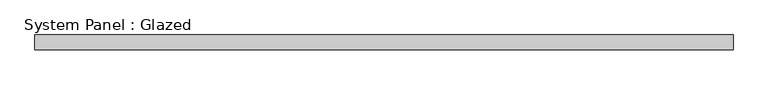
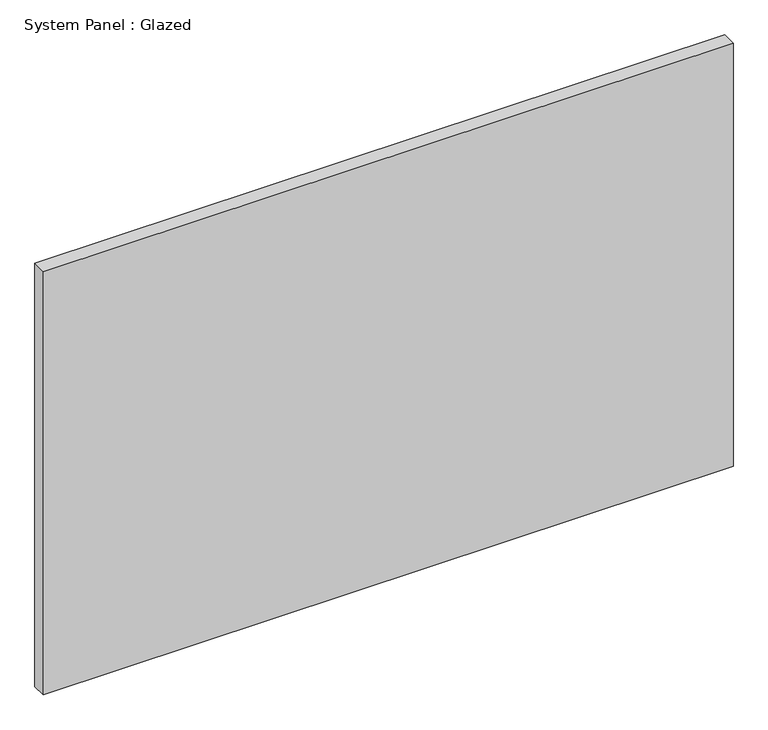
"""IFC4 building model written with IfcOpenShell, lengths in millimetres: plate geometry, System Panel : Glazed."""

from ifc_helpers import new_model, si_unit, origin, origin_with_axes, place, context, project, spatial, polyline, outline, extrude, source, transform, mapped, element, save


def system_panel_glazed_7a6fc0cf(model_context):
    return source(origin(), model_context, "Body", "SweptSolid", [
        extrude(outline(polyline([(604.6949353, 19.05), (-604.6949353, 19.05), (-604.6949353, 44.45), (604.6949353, 44.45), (604.6949353, 19.05)])), origin_with_axes(), (0.0, 0.0, 1.0), 784.5104839),
    ])


if __name__ == "__main__":
    model = new_model("IFC4")
    model_context = context("Model", 3, world=origin())
    ifc_project = project(units=[si_unit("LENGTHUNIT", "METRE", prefix="MILLI")], contexts=[model_context])
    site = spatial("IfcSite", under=ifc_project)
    building = spatial("IfcBuilding", under=site)
    placement = place(None, origin())
    system_panel_glazed_shape = system_panel_glazed_7a6fc0cf(model_context)
    element("IfcPlate", 1, ObjectType="System Panel : Glazed", at=placement, inside=building, context=model_context, shape_type="MappedRepresentation", body=[
        mapped(system_panel_glazed_shape, transform((0.0, 0.0, 0.0), x_axis=(1.0, 0.0, 0.0), y_axis=(0.0, 1.0, 0.0), z_axis=(0.0, 0.0, 1.0))),
    ])
    save(model, "model.ifc")

# Revit data of these elements
# Type "System Panel : Glazed"
#   Construction Type Id = "GSP4R"
#   Analytic Construction = "1/8 in Pilkington single glazing"
#   Visual Light Transmittance = 0.9
#   Solar Heat Gain Coefficient = 0.86
#   Heat Transfer Coefficient (U) = 1.18115 BTU/(h·ft²·°F)
#   Define Thermal Properties by = 1
# Element 1 (IfcPlate, "System Panel : Glazed")
#   Materials on its faces: "Glass"
# Materials
#   "Glass": class "Glass", colour RGB 0 128 192, transparency 0.75, Description = "Soda Lime Glass", Cost = 0
